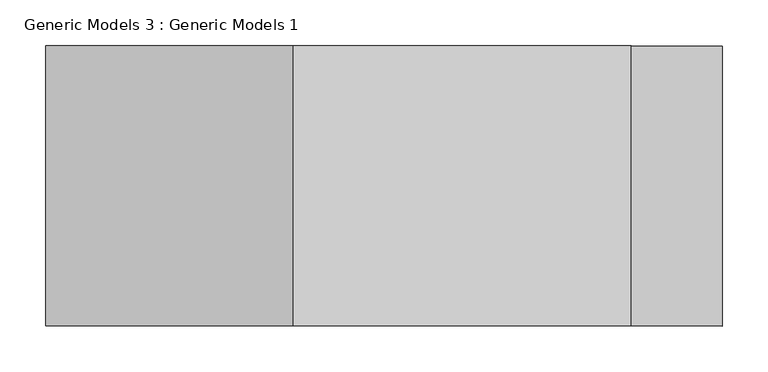
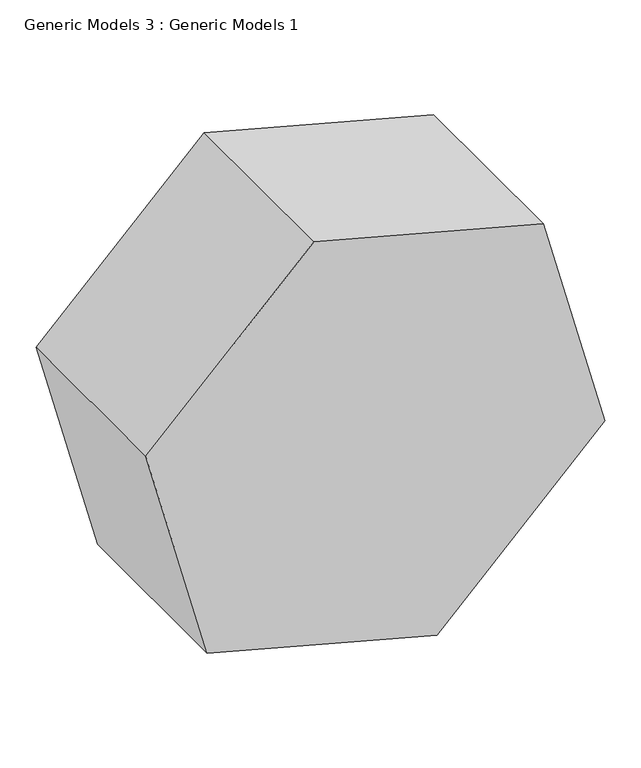
"""IFC4 building model written with IfcOpenShell, lengths in millimetres: proxy geometry, Generic Models 3 : Generic Models 1."""

from ifc_helpers import new_model, si_unit, frame, origin, place, context, project, spatial, polyline, outline, extrude, source, transform, mapped, element, save


def generic_models_3_generic_models_1_c8895c90(model_context):
    return source(origin(), model_context, "Body", "SweptSolid", [
        extrude(outline(polyline([(904.7566299, -8120.6070438), (1003.366686, -8488.6247836), (733.9590024, -8758.0324672), (365.9412626, -8659.422411), (267.3312064, -8291.4046712), (536.73889, -8021.9969876), (904.7566299, -8120.6070438)])), frame((0.0, -9086.6225464, 0.0), z_axis=(0.0, 1.0, 0.0), x_axis=(0.0, 0.0, 1.0)), (0.0, 0.0, 1.0), 304.8),
    ])


if __name__ == "__main__":
    model = new_model("IFC4")
    model_context = context("Model", 3, world=origin())
    ifc_project = project(units=[si_unit("LENGTHUNIT", "METRE", prefix="MILLI")], contexts=[model_context])
    site = spatial("IfcSite", under=ifc_project)
    building = spatial("IfcBuilding", under=site)
    placement = place(None, origin())
    generic_models_3_generic_models_1_shape = generic_models_3_generic_models_1_c8895c90(model_context)
    element("IfcBuildingElementProxy", 1, Name="Generic Models 3 : Generic Models 1", ObjectType="Generic Models 3 : Generic Models 1", at=placement, inside=building, context=model_context, shape_type="MappedRepresentation", body=[
        mapped(generic_models_3_generic_models_1_shape, transform((0.0, 0.0, 0.0), x_axis=(1.0, 0.0, 0.0), y_axis=(0.0, 1.0, 0.0), z_axis=(0.0, 0.0, 1.0))),
    ])
    save(model, "model.ifc")

# Revit data of these elements
# Element 1 (IfcBuildingElementProxy, "Generic Models 3 : Generic Models 1")
#   Materials on its faces: "Carpet (1)"
# Materials
#   "Carpet (1)": class "Carpet", colour RGB 124 80 67, transparency 0, Description = "Interior finish", Cost = 0
